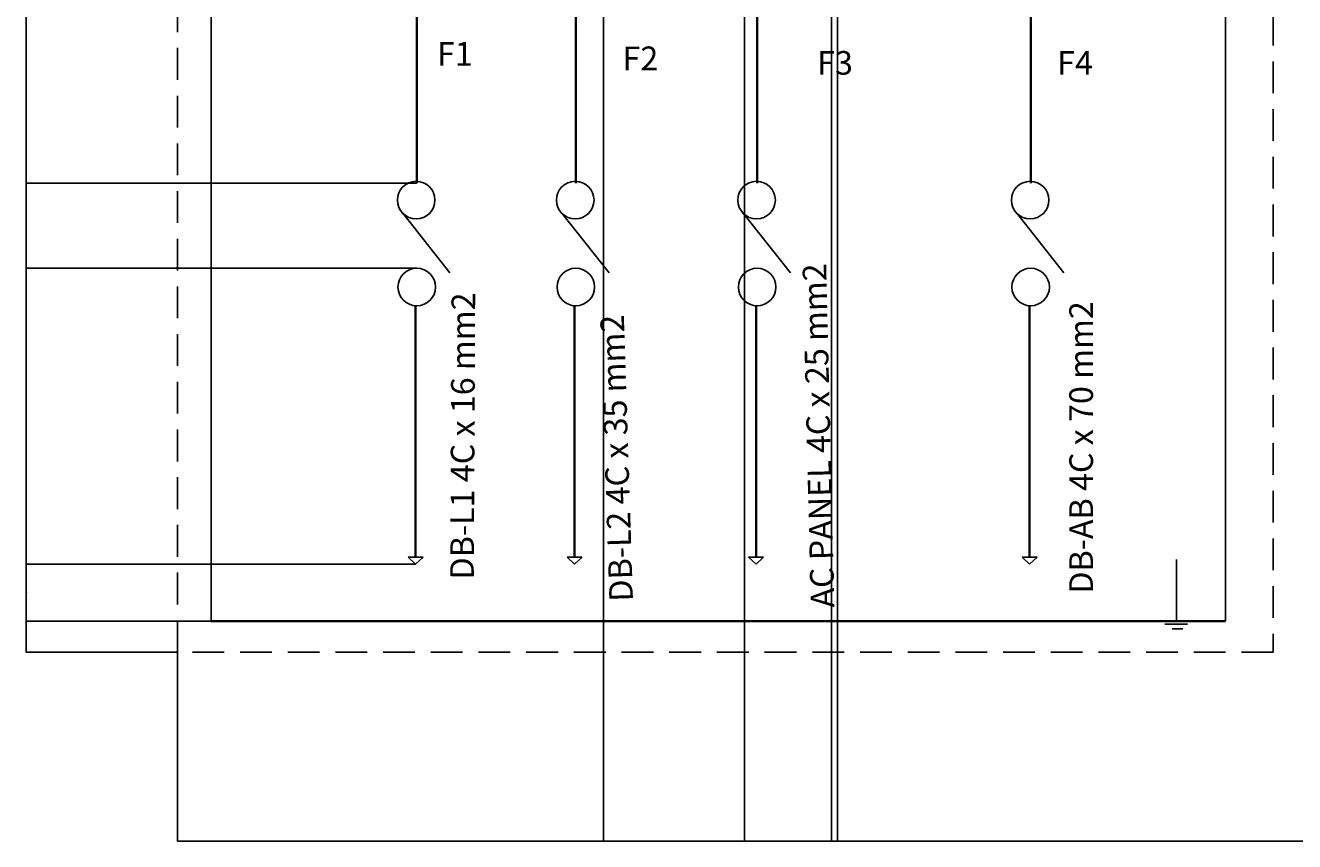
# Model space of a CAD drawing. Units: millimetres. Extents: x 1832 to 3146, y 927 to 1751.
# Tile 1 of 4: x 1832 to 2339, y 927 to 1253. Entities that reach past the tile are written whole.
import ezdxf

# ---------------------------------------------------------------- set-up
doc = ezdxf.new("R2010")
doc.units = ezdxf.units.MM
doc.header["$MEASUREMENT"] = 0
doc.linetypes.add('DASHED', pattern=[19.05, 12.7, -6.35])
doc.layers.get('0').update_dxf_attribs({"color": 2, "lineweight": 35})
doc.layers.get('0').transparency = 0.01
for name, color, linetype, lineweight in [('A-ANNO-DIMS', 2, 'Continuous', 18), ('E-ANNO-TEXT', 7, 'Continuous', 18), ('E-POWR-EQPM', 2, 'Continuous', 25), ('E-POWR-PNLS', 3, 'DASHED', 25), ('E-POWR-WIRE', 7, 'Continuous', 35)]:
    doc.layers.add(name, color=color, linetype=linetype, lineweight=lineweight)
doc.styles.get("Standard").update_dxf_attribs({"font": 'arial.ttf'})
doc.dimstyles.get("Standard").update_dxf_attribs({"dimtxt": 0.18, "dimasz": 0.18, "dimexe": 0.18, "dimexo": 0.0625, "dimgap": 0.09, "dimtad": 0, "dimtih": 1, "dimtoh": 1, "dimdec": 4, "dimzin": 0, "dimdsep": 46, "dimtxsty": 'Standard', "dimcen": 0.09, "dimadec": 0, "dimazin": 0, "dimtfac": 1, "dimtdec": 4, "dimtofl": 0, "dimtmove": 0, "dimatfit": 3, "dimfxl": 1, "dimtolj": 1, "dimtzin": 0, "dimarcsym": 0})

# ---------------------------------------------------------------- blocks, each defined once
blk = doc.blocks.new('CB-FEEDER')
blk.add_line((1982.97, 1178.23), (2001.83, 1154.39))
for points in [[(1980.83, 1183.48, 1), (1995.83, 1183.48, 1)], [(1981.05, 1148.75, 1), (1996.05, 1148.75, 1)]]:
    blk.add_lwpolyline(points, format="xyb", close=True)
blk = doc.blocks.new('CABLE-ARROW')
for p, q in [((1988.1, 1040.89), (1985.1, 1040.84)), ((1985.1, 1040.84), (1988.1, 1038.05)), ((1988.1, 1040.89), (1991.1, 1040.89)), ((1991.1, 1040.89), (1988.1, 1038.05))]:
    blk.add_line(p, q)
blk = doc.blocks.new('*D9')
at = {"layer": 'A-ANNO-DIMS', "color": 0, "lineweight": -2, "transparency": 16777216}
for p, q in [((1892.94, 1002.86), (1892.94, 927.26)), ((3085.33, 987.73), (3085.33, 927.26)), ((1893.12, 927.44), (2488.68, 927.44)), ((3085.15, 927.44), (2489.59, 927.44))]:
    blk.add_line(p, q, dxfattribs=at)
at = {"layer": 'A-ANNO-DIMS', "color": 0, "lineweight": 35, "transparency": 16777216}
for points in [[(1893.12, 927.47), (1893.12, 927.41), (1892.94, 927.44)], [(3085.15, 927.47), (3085.15, 927.41), (3085.33, 927.44)]]:
    blk.add_solid(points, dxfattribs=at)
at = {"layer": 'Defpoints', "color": 0, "lineweight": 35, "transparency": 16777216}
for p in [(1892.94, 1002.93), (3085.33, 987.79), (3085.33, 927.44)]:
    blk.add_point(p, dxfattribs=at)
at = {"layer": 'A-ANNO-DIMS', "color": 0, "transparency": 16777216, "insert": (2489.13, 927.44), "char_height": 0.18, "attachment_point": 5}
blk.add_mtext('\\A1;1192.4', dxfattribs=at)
blk = doc.blocks.new('*D11')
at = {"layer": 'A-ANNO-DIMS', "color": 0, "lineweight": -2, "transparency": 16777216}
for p, q in [((1892.88, 1334.1), (1832.41, 1334.1)), ((1832.59, 1333.92), (1832.59, 1168.69)), ((1832.59, 1003.11), (1832.59, 1168.33)), ((1892.88, 1002.93), (1832.41, 1002.93))]:
    blk.add_line(p, q, dxfattribs=at)
at = {"layer": 'A-ANNO-DIMS', "color": 0, "lineweight": 35, "transparency": 16777216}
for points in [[(1832.56, 1333.92), (1832.62, 1333.92), (1832.59, 1334.1)], [(1832.56, 1003.11), (1832.62, 1003.11), (1832.59, 1002.93)]]:
    blk.add_solid(points, dxfattribs=at)
at = {"layer": 'Defpoints', "color": 0, "lineweight": 35, "transparency": 16777216}
for p in [(1832.59, 1334.1), (1892.94, 1334.1), (1892.94, 1002.93)]:
    blk.add_point(p, dxfattribs=at)
at = {"layer": 'A-ANNO-DIMS', "color": 0, "transparency": 16777216, "insert": (1832.59, 1168.51), "char_height": 0.18, "attachment_point": 5}
blk.add_mtext('\\A1;331.2', dxfattribs=at)
blk = doc.blocks.new('*D27')
at = {"layer": 'A-ANNO-DIMS', "color": 0, "lineweight": -2, "transparency": 16777216}
for p, q in [((1906.41, 1015.38), (1906.41, 1750.84)), ((1906.59, 1750.66), (2108.57, 1750.66)), ((2311.47, 1750.66), (2109.5, 1750.66)), ((2311.65, 1015.38), (2311.65, 1750.84))]:
    blk.add_line(p, q, dxfattribs=at)
at = {"layer": 'A-ANNO-DIMS', "color": 0, "lineweight": 35, "transparency": 16777216}
for points in [[(1906.59, 1750.69), (1906.59, 1750.63), (1906.41, 1750.66)], [(2311.47, 1750.69), (2311.47, 1750.63), (2311.65, 1750.66)]]:
    blk.add_solid(points, dxfattribs=at)
at = {"layer": 'Defpoints', "color": 0, "lineweight": 35, "transparency": 16777216}
for p in [(2311.65, 1750.66), (1906.41, 1015.32), (2311.65, 1015.32)]:
    blk.add_point(p, dxfattribs=at)
at = {"layer": 'A-ANNO-DIMS', "color": 0, "transparency": 16777216, "insert": (2109.03, 1750.66), "char_height": 0.18, "attachment_point": 5}
blk.add_mtext('\\A1;405.24', dxfattribs=at)
blk = doc.blocks.new('*D32')
at = {"layer": 'A-ANNO-DIMS', "color": 0, "lineweight": -2, "transparency": 16777216}
for p, q in [((2063.17, 1685.25), (2063.17, 927.26)), ((2154.3, 1685.25), (2154.3, 927.26)), ((2063.35, 927.44), (2108.34, 927.44)), ((2154.12, 927.44), (2109.13, 927.44))]:
    blk.add_line(p, q, dxfattribs=at)
at = {"layer": 'A-ANNO-DIMS', "color": 0, "lineweight": 35, "transparency": 16777216}
for points in [[(2063.35, 927.47), (2063.35, 927.41), (2063.17, 927.44)], [(2154.12, 927.47), (2154.12, 927.41), (2154.3, 927.44)]]:
    blk.add_solid(points, dxfattribs=at)
at = {"layer": 'Defpoints', "color": 0, "lineweight": 35, "transparency": 16777216}
for p in [(2063.17, 1685.32), (2154.3, 1685.32), (2154.3, 927.44)]:
    blk.add_point(p, dxfattribs=at)
at = {"layer": 'A-ANNO-DIMS', "color": 0, "transparency": 16777216, "insert": (2108.74, 927.44), "char_height": 0.18, "attachment_point": 5}
blk.add_mtext('\\A1;91.13', dxfattribs=at)
blk = doc.blocks.new('*D34')
at = {"layer": 'A-ANNO-DIMS', "color": 0, "lineweight": -2, "transparency": 16777216}
for p, q in [((2119.54, 1640.76), (2119.54, 927.26)), ((2156.63, 1634.27), (2156.63, 927.26)), ((2119.72, 927.44), (2137.69, 927.44)), ((2156.45, 927.44), (2138.48, 927.44))]:
    blk.add_line(p, q, dxfattribs=at)
at = {"layer": 'A-ANNO-DIMS', "color": 0, "lineweight": 35, "transparency": 16777216}
for points in [[(2119.72, 927.47), (2119.72, 927.41), (2119.54, 927.44)], [(2156.45, 927.47), (2156.45, 927.41), (2156.63, 927.44)]]:
    blk.add_solid(points, dxfattribs=at)
at = {"layer": 'Defpoints', "color": 0, "lineweight": 35, "transparency": 16777216}
for p in [(2119.54, 1640.82), (2156.63, 1634.33), (2156.63, 927.44)]:
    blk.add_point(p, dxfattribs=at)
at = {"layer": 'A-ANNO-DIMS', "color": 0, "transparency": 16777216, "insert": (2138.08, 927.44), "char_height": 0.18, "attachment_point": 5}
blk.add_mtext('\\A1;37.10', dxfattribs=at)
blk = doc.blocks.new('*D42')
at = {"layer": 'A-ANNO-DIMS', "color": 0, "lineweight": -2, "transparency": 16777216}
for p, q in [((1988.49, 1259.88), (1832.41, 1259.88)), ((1832.59, 1259.7), (1832.59, 1225.24)), ((1832.59, 1190.42), (1832.59, 1224.88)), ((1988.49, 1190.24), (1832.41, 1190.24))]:
    blk.add_line(p, q, dxfattribs=at)
at = {"layer": 'A-ANNO-DIMS', "color": 0, "lineweight": 35, "transparency": 16777216}
for points in [[(1832.56, 1259.7), (1832.62, 1259.7), (1832.59, 1259.88)], [(1832.56, 1190.42), (1832.62, 1190.42), (1832.59, 1190.24)]]:
    blk.add_solid(points, dxfattribs=at)
at = {"layer": 'Defpoints', "color": 0, "lineweight": 35, "transparency": 16777216}
for p in [(1988.55, 1259.88), (1832.59, 1190.24), (1988.55, 1190.24)]:
    blk.add_point(p, dxfattribs=at)
at = {"layer": 'A-ANNO-DIMS', "color": 0, "transparency": 16777216, "insert": (1832.59, 1225.06), "char_height": 0.18, "attachment_point": 5}
blk.add_mtext('\\A1;69.64', dxfattribs=at)
blk = doc.blocks.new('*D43')
at = {"layer": 'A-ANNO-DIMS', "color": 0, "lineweight": -2, "transparency": 16777216}
for p, q in [((1988.49, 1190.24), (1832.41, 1190.24)), ((1832.59, 1190.06), (1832.59, 1173.43)), ((1832.59, 1156.43), (1832.59, 1173.07)), ((1988.49, 1156.25), (1832.41, 1156.25))]:
    blk.add_line(p, q, dxfattribs=at)
at = {"layer": 'A-ANNO-DIMS', "color": 0, "lineweight": 35, "transparency": 16777216}
for points in [[(1832.56, 1190.06), (1832.62, 1190.06), (1832.59, 1190.24)], [(1832.56, 1156.43), (1832.62, 1156.43), (1832.59, 1156.25)]]:
    blk.add_solid(points, dxfattribs=at)
at = {"layer": 'Defpoints', "color": 0, "lineweight": 35, "transparency": 16777216}
for p in [(1988.55, 1190.24), (1832.59, 1156.25), (1988.55, 1156.25)]:
    blk.add_point(p, dxfattribs=at)
at = {"layer": 'A-ANNO-DIMS', "color": 0, "transparency": 16777216, "insert": (1832.59, 1173.25), "char_height": 0.18, "attachment_point": 5}
blk.add_mtext('\\A1;33.99', dxfattribs=at)
blk = doc.blocks.new('*D44')
at = {"layer": 'A-ANNO-DIMS', "color": 0, "lineweight": -2, "transparency": 16777216}
for p, q in [((1988.49, 1156.25), (1832.41, 1156.25)), ((1832.59, 1156.07), (1832.59, 1097.34)), ((1832.59, 1038.23), (1832.59, 1096.97)), ((1988.04, 1038.05), (1832.41, 1038.05))]:
    blk.add_line(p, q, dxfattribs=at)
at = {"layer": 'A-ANNO-DIMS', "color": 0, "lineweight": 35, "transparency": 16777216}
for points in [[(1832.56, 1156.07), (1832.62, 1156.07), (1832.59, 1156.25)], [(1832.56, 1038.23), (1832.62, 1038.23), (1832.59, 1038.05)]]:
    blk.add_solid(points, dxfattribs=at)
at = {"layer": 'Defpoints', "color": 0, "lineweight": 35, "transparency": 16777216}
for p in [(1988.55, 1156.25), (1832.59, 1038.05), (1988.1, 1038.05)]:
    blk.add_point(p, dxfattribs=at)
at = {"layer": 'A-ANNO-DIMS', "color": 0, "transparency": 16777216, "insert": (1832.59, 1097.15), "char_height": 0.18, "attachment_point": 5}
blk.add_mtext('\\A1;118.20', dxfattribs=at)
blk = doc.blocks.new('*D45')
at = {"layer": 'A-ANNO-DIMS', "color": 0, "lineweight": -2, "transparency": 16777216}
for p, q in [((1988.04, 1038.05), (1832.41, 1038.05)), ((1832.59, 1037.87), (1832.59, 1026.87)), ((1832.59, 1015.5), (1832.59, 1026.51)), ((1906.35, 1015.32), (1832.41, 1015.32))]:
    blk.add_line(p, q, dxfattribs=at)
at = {"layer": 'A-ANNO-DIMS', "color": 0, "lineweight": 35, "transparency": 16777216}
for points in [[(1832.56, 1037.87), (1832.62, 1037.87), (1832.59, 1038.05)], [(1832.56, 1015.5), (1832.62, 1015.5), (1832.59, 1015.32)]]:
    blk.add_solid(points, dxfattribs=at)
at = {"layer": 'Defpoints', "color": 0, "lineweight": 35, "transparency": 16777216}
for p in [(1988.1, 1038.05), (1832.59, 1015.32), (1906.41, 1015.32)]:
    blk.add_point(p, dxfattribs=at)
at = {"layer": 'A-ANNO-DIMS', "color": 0, "transparency": 16777216, "insert": (1832.59, 1026.69), "char_height": 0.18, "attachment_point": 5}
blk.add_mtext('\\A1;22.732', dxfattribs=at)

msp = doc.modelspace()

# ---------------------------------------------------------------- linework, layer by layer
at = {"layer": 'E-POWR-EQPM'}
for p, q in [((2292.0646, 1015.321), (2292.0646, 1039.9441)), ((2287.4295, 1014.0742), (2296.4634, 1014.0742)), ((2290.3179, 1012.2321), (2294.5583, 1012.2321))]:
    msp.add_line(p, q, dxfattribs=at)
at = {"layer": 'E-POWR-PNLS'}
msp.add_lwpolyline([(1892.9387, 1334.0963), (2330.7306, 1334.0963), (2330.7306, 1002.9254), (1892.9387, 1002.9254)], close=True, dxfattribs=at)
at = {"layer": 'E-POWR-WIRE'}
for p, q in [((1988.5483, 1259.8778), (1988.5483, 1190.2428)), ((2052.0805, 1259.8778), (2052.0805, 1190.2428)), ((2124.5321, 1259.8778), (2124.5321, 1190.2428)), ((2233.8033, 1259.8778), (2233.8033, 1190.2428)), ((1988.0989, 1141.267), (1988.0989, 1040.8938)), ((2051.6312, 1141.267), (2051.6312, 1040.8938)), ((2124.0827, 1141.267), (2124.0827, 1040.8938)), ((2233.354, 1141.267), (2233.354, 1040.8938)), ((1906.4128, 1015.321), (2311.6539, 1015.321))]:
    msp.add_line(p, q, dxfattribs=at)

# ---------------------------------------------------------------- block references
at = {"layer": 'E-POWR-EQPM'}
for name, p in [('CB-FEEDER', (0, 0)), ('CB-FEEDER', (63.5323, 0)), ('CB-FEEDER', (135.9839, 0)), ('CB-FEEDER', (245.2551, 0)), ('CABLE-ARROW', (0, 0)), ('CABLE-ARROW', (63.5323, 0)), ('CABLE-ARROW', (135.9839, 0)), ('CABLE-ARROW', (245.2551, 0))]:
    msp.add_blockref(name, p, dxfattribs=at)

# ---------------------------------------------------------------- texts
at = {"layer": 'E-ANNO-TEXT'}
for s, p in [('F1', (1996.6267, 1237.1618)), ('F2', (2070.7736, 1235.355)), ('F3', (2148.5375, 1233.5481)), ('F4', (2244.3859, 1233.5481))]:
    msp.add_text(s, height=9.44797, dxfattribs=at).set_placement(p)
for s, rotation, p in [('AC PANEL 4C x 25 mm2', 91.382689, (2155.41, 1020.8161)), ('DB-L1 4C x 16 mm2', 89.717716, (2011.3504, 1031.927)), ('DB-AB 4C x 70 mm2', 90, (2258.6848, 1026.2831)), ('DB-L2 4C x 35 mm2', 91.837034, (2074.9525, 1023.2369))]:
    msp.add_text(s, height=9.447971, rotation=rotation, dxfattribs=at).set_placement(p)

# ---------------------------------------------------------------- dimensions: what is measured, and where the dimension line sits
at = {"layer": 'A-ANNO-DIMS'}
for base, p1, p2, override, picture, middle in [((2311.6539, 1750.6609), (1906.4128, 1015.321), (2311.6539, 1015.321), {"dimdec": 2, "dimlfac": 1, "dimrnd": 0, "dimzin": 0, "dimdsep": 46, "dimlunit": 2}, '*D27', (2109.0334, 1750.6609)), ((2154.2992, 927.4392), (2063.171, 1685.3164), (2154.2992, 1685.3164), {"dimdec": 2, "dimlfac": 1, "dimrnd": 0, "dimzin": 0, "dimdsep": 46, "dimlunit": 2}, '*D32', (2108.7351, 927.4392)), ((2156.6335, 927.4392), (2119.5362, 1640.8227), (2156.6335, 1634.3311), {"dimdec": 2, "dimlfac": 1, "dimrnd": 0, "dimzin": 0, "dimdsep": 46, "dimlunit": 2}, '*D34', (2138.0848, 927.4392)), ((3085.3254, 927.4392), (1892.9387, 1002.9254), (3085.3254, 987.7892), {"dimdec": 1, "dimlfac": 1, "dimrnd": 0, "dimzin": 0, "dimdsep": 46, "dimlunit": 2}, '*D9', (2489.1321, 927.4392))]:
    dim = msp.add_linear_dim(base=base, p1=p1, p2=p2, dimstyle='Standard', override=override, dxfattribs=at)
    dim.commit()
    dim.dimension.update_dxf_attribs({"geometry": picture, "text_midpoint": middle})
for base, p1, p2, override, picture, middle in [((1832.5887, 1334.0963), (1892.9387, 1002.9254), (1892.9387, 1334.0963), {"dimdec": 1, "dimlfac": 1, "dimrnd": 0, "dimzin": 0, "dimdsep": 46, "dimlunit": 2}, '*D11', (1832.5887, 1168.5109)), ((1832.58868, 1190.24279), (1988.54826, 1259.87783), (1988.54826, 1190.24279), {"dimdec": 2, "dimlfac": 1, "dimrnd": 0, "dimzin": 0, "dimdsep": 46, "dimlunit": 2}, '*D42', (1832.58868, 1225.06031)), ((1832.5887, 1156.2535), (1988.5483, 1190.2428), (1988.5483, 1156.2535), {"dimdec": 2, "dimlfac": 1, "dimrnd": 0, "dimzin": 0, "dimdsep": 46, "dimlunit": 2}, '*D43', (1832.5887, 1173.2481)), ((1832.5887, 1038.0533), (1988.5483, 1156.2535), (1988.0989, 1038.0533), {"dimdec": 2, "dimlfac": 1, "dimrnd": 0, "dimzin": 0, "dimdsep": 46, "dimlunit": 2}, '*D44', (1832.5887, 1097.1534)), ((1832.5887, 1015.321), (1988.0989, 1038.0533), (1906.4128, 1015.321), {"dimdec": 3, "dimlfac": 1, "dimrnd": 0, "dimzin": 0, "dimdsep": 46, "dimlunit": 2}, '*D45', (1832.5887, 1026.6871))]:
    dim = msp.add_linear_dim(base=base, p1=p1, p2=p2, angle=90, dimstyle='Standard', override=override, dxfattribs=at)
    dim.commit()
    dim.dimension.update_dxf_attribs({"geometry": picture, "text_midpoint": middle})

doc.saveas('drawing.dxf')
